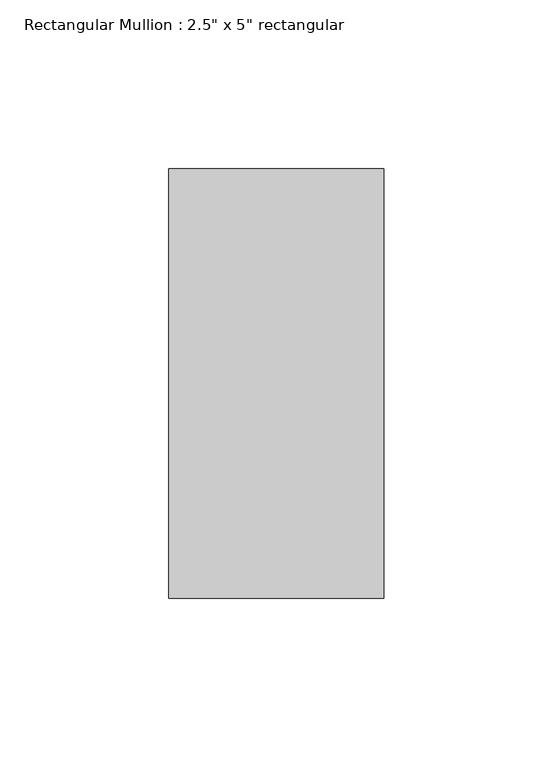
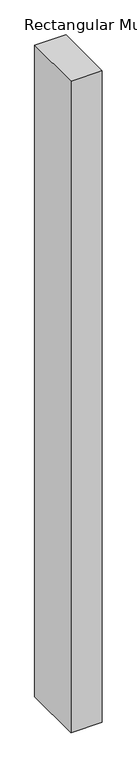
"""IFC4 building model written with IfcOpenShell, lengths in millimetres: member geometry."""

from ifc_helpers import new_model, si_unit, frame, origin, place, context, project, spatial, polyline, outline, extrude, source, transform, mapped, element, save


def member_d72f1a08(model_context):
    return source(origin(), model_context, "Body", "SweptSolid", [
        extrude(outline(polyline([(31.75, 63.5), (31.75, -63.5), (-31.75, -63.5), (-31.75, 63.5), (31.75, 63.5)])), frame((0.0, 0.0, -1397.2284812), z_axis=(0.0, 0.0, 1.0), x_axis=(1.0, 0.0, 0.0)), (0.0, 0.0, 1.0), 1397.2284812),
    ])


if __name__ == "__main__":
    model = new_model("IFC4")
    model_context = context("Model", 3, world=origin())
    ifc_project = project(units=[si_unit("LENGTHUNIT", "METRE", prefix="MILLI")], contexts=[model_context])
    site = spatial("IfcSite", under=ifc_project)
    building = spatial("IfcBuilding", under=site)
    placement = place(None, origin())
    member_shape = member_d72f1a08(model_context)
    element("IfcMember", 1, ObjectType="Rectangular Mullion : 2.5\" x 5\" rectangular", at=placement, inside=building, context=model_context, shape_type="MappedRepresentation", body=[
        mapped(member_shape, transform((0.0, 0.0, 0.0), x_axis=(1.0, 0.0, 0.0), y_axis=(0.0, 1.0, 0.0), z_axis=(0.0, 0.0, 1.0))),
    ])
    save(model, "model.ifc")

# Revit data of these elements
# Type "Rectangular Mullion : 2.5\" x 5\" rectangular"
#   built-in parameter 1007304 = 0.416667 (stored number, unit not read)
#   built-in parameter 1007301 = 0.104167 (stored number, unit not read)
#   built-in parameter 1007300 = 0.104167 (stored number, unit not read)
# Element 1 (IfcMember, "Rectangular Mullion : 2.5\" x 5\" rectangular")
#   Materials on its faces: "Aluminum"
# Materials
#   "Aluminum": class "Metal", colour RGB 247 247 247, transparency 0, Description = "Aluminum 6061", Cost = 0
